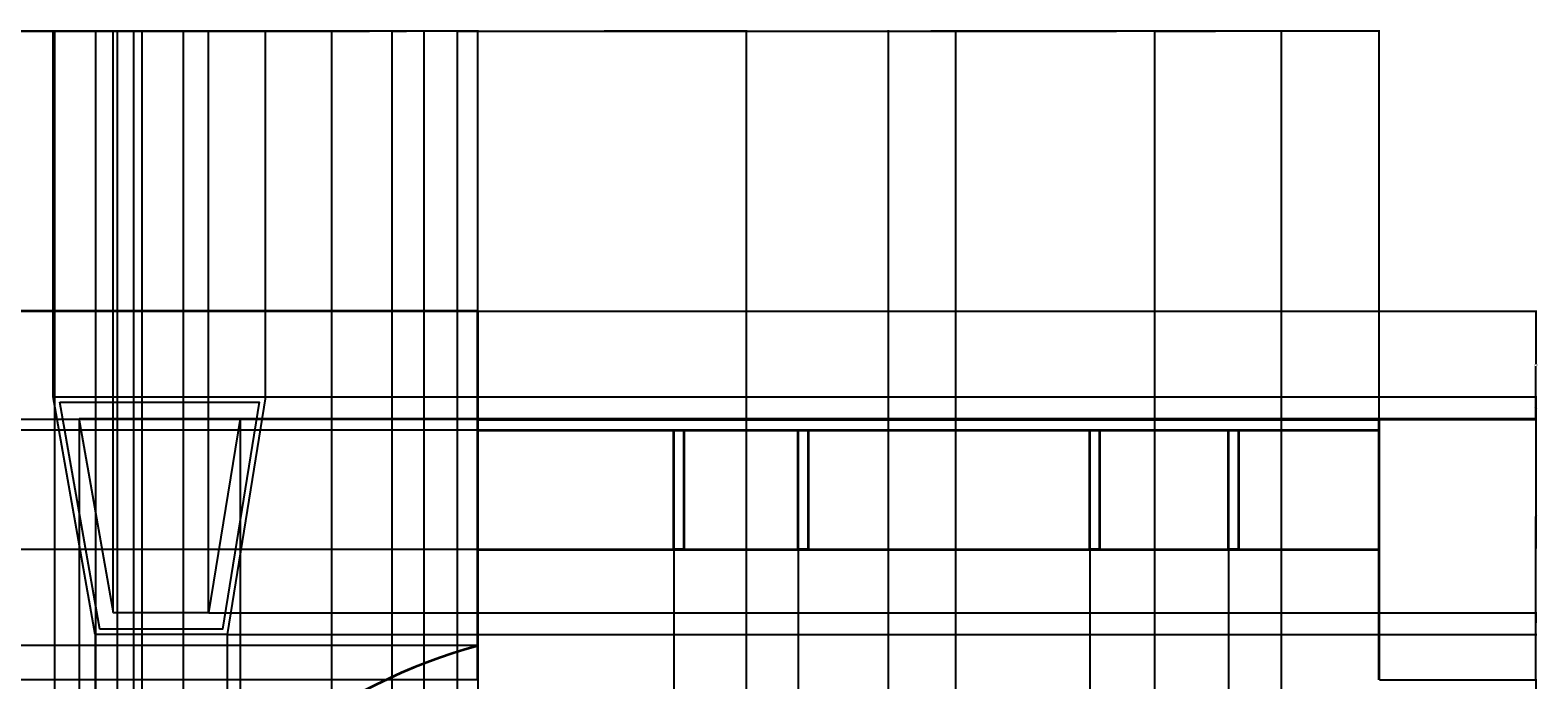
# Model space of a CAD drawing. Units: inches. Extents: x -19 to 408, y -26 to 603.
# Tile 7 of 7: x 130 to 408, y 483 to 603. Entities that reach past the tile are written whole.
import ezdxf

# ---------------------------------------------------------------- set-up
doc = ezdxf.new("R2010")
doc.units = ezdxf.units.IN
doc.header["$MEASUREMENT"] = 0
for name, color, linetype, lineweight in [('A-ANNO-DIMS', 2, 'Continuous', 18), ('A-ELEV', 7, 'Continuous', 35), ('A-GLAZ', 4, 'Continuous', 25)]:
    doc.layers.add(name, color=color, linetype=linetype, lineweight=lineweight)
doc.styles.get("Standard").update_dxf_attribs({"font": 'arial.ttf'})
doc.dimstyles.get("Standard").update_dxf_attribs({"dimtxt": 0.18, "dimasz": 0.18, "dimexe": 0.18, "dimexo": 0.0625, "dimgap": 0.09, "dimtad": 0, "dimtih": 1, "dimtoh": 1, "dimdec": 4, "dimzin": 0, "dimdsep": 46, "dimtxsty": 'Standard', "dimcen": 0.09, "dimadec": 0, "dimazin": 0, "dimtfac": 1, "dimtdec": 4, "dimtofl": 0, "dimtmove": 0, "dimatfit": 3, "dimfxl": 1, "dimtolj": 1, "dimtzin": 0, "dimarcsym": 0})

# ---------------------------------------------------------------- blocks, each defined once
blk = doc.blocks.new('RAIL-POST')
blk.add_lwpolyline([(0, 22), (1.83, 22), (1.83, 0), (0, 0)], close=True)
blk = doc.blocks.new('*D15')
at = {"layer": 'A-ANNO-DIMS', "color": 0, "lineweight": -2, "transparency": 16777216}
for p, q in [((10.2, 573.88), (10.2, 602.9)), ((10.38, 602.72), (110.85, 602.72)), ((212.25, 602.72), (111.78, 602.72)), ((212.43, 551.17), (212.43, 602.9))]:
    blk.add_line(p, q, dxfattribs=at)
at = {"layer": 'A-ANNO-DIMS', "color": 0, "transparency": 16777216}
for points in [[(10.38, 602.75), (10.38, 602.69), (10.2, 602.72)], [(212.25, 602.75), (212.25, 602.69), (212.43, 602.72)]]:
    blk.add_solid(points, dxfattribs=at)
at = {"layer": 'Defpoints', "color": 0, "transparency": 16777216}
for p in [(212.43, 602.72), (10.2, 573.82), (212.43, 551.1)]:
    blk.add_point(p, dxfattribs=at)
at = {"layer": 'A-ANNO-DIMS', "color": 0, "transparency": 16777216, "insert": (111.32, 602.72), "char_height": 0.18, "attachment_point": 5}
blk.add_mtext('\\A1;202.23', dxfattribs=at)
blk = doc.blocks.new('*D16')
at = {"layer": 'A-ANNO-DIMS', "color": 0, "lineweight": -2, "transparency": 16777216}
for p, q in [((212.43, 551.17), (212.43, 602.9)), ((212.61, 602.72), (295.05, 602.72)), ((378.39, 602.72), (295.96, 602.72)), ((378.57, 531.21), (378.57, 602.9))]:
    blk.add_line(p, q, dxfattribs=at)
at = {"layer": 'A-ANNO-DIMS', "color": 0, "transparency": 16777216}
for points in [[(212.61, 602.75), (212.61, 602.69), (212.43, 602.72)], [(378.39, 602.75), (378.39, 602.69), (378.57, 602.72)]]:
    blk.add_solid(points, dxfattribs=at)
at = {"layer": 'Defpoints', "color": 0, "transparency": 16777216}
for p in [(378.57, 602.72), (212.43, 551.1), (378.57, 531.15)]:
    blk.add_point(p, dxfattribs=at)
at = {"layer": 'A-ANNO-DIMS', "color": 0, "transparency": 16777216, "insert": (295.5, 602.72), "char_height": 0.18, "attachment_point": 5}
blk.add_mtext('\\A1;166.14', dxfattribs=at)
blk = doc.blocks.new('*D21')
at = {"layer": 'A-ANNO-DIMS', "color": 0, "lineweight": -2, "transparency": 16777216}
for p, q in [((212.37, 551.1), (-18.88, 551.1)), ((-18.7, 550.92), (-18.7, 481.31)), ((-18.7, 411.33), (-18.7, 480.94)), ((185.46, 411.15), (-18.88, 411.15))]:
    blk.add_line(p, q, dxfattribs=at)
at = {"layer": 'A-ANNO-DIMS', "color": 0, "transparency": 16777216}
for points in [[(-18.73, 550.92), (-18.67, 550.92), (-18.7, 551.1)], [(-18.73, 411.33), (-18.67, 411.33), (-18.7, 411.15)]]:
    blk.add_solid(points, dxfattribs=at)
at = {"layer": 'Defpoints', "color": 0, "transparency": 16777216}
for p in [(-18.7, 551.1), (212.43, 551.1), (185.52, 411.15)]:
    blk.add_point(p, dxfattribs=at)
at = {"layer": 'A-ANNO-DIMS', "color": 0, "transparency": 16777216, "insert": (-18.7, 481.13), "char_height": 0.18, "attachment_point": 5}
blk.add_mtext('\\A1;139.96', dxfattribs=at)
blk = doc.blocks.new('*D22')
at = {"layer": 'A-ANNO-DIMS', "color": 0, "lineweight": -2, "transparency": 16777216}
for p, q in [((10.14, 573.82), (-18.88, 573.82)), ((-18.7, 573.64), (-18.7, 562.64)), ((-18.7, 551.28), (-18.7, 562.28)), ((212.37, 551.1), (-18.88, 551.1))]:
    blk.add_line(p, q, dxfattribs=at)
at = {"layer": 'A-ANNO-DIMS', "color": 0, "transparency": 16777216}
for points in [[(-18.73, 573.64), (-18.67, 573.64), (-18.7, 573.82)], [(-18.73, 551.28), (-18.67, 551.28), (-18.7, 551.1)]]:
    blk.add_solid(points, dxfattribs=at)
at = {"layer": 'Defpoints', "color": 0, "transparency": 16777216}
for p in [(-18.7, 573.82), (10.2, 573.82), (212.43, 551.1)]:
    blk.add_point(p, dxfattribs=at)
at = {"layer": 'A-ANNO-DIMS', "color": 0, "transparency": 16777216, "insert": (-18.7, 562.46), "char_height": 0.18, "attachment_point": 5}
blk.add_mtext('\\A1;22.714', dxfattribs=at)
blk = doc.blocks.new('*D24')
at = {"layer": 'A-ANNO-DIMS', "color": 0, "lineweight": -2, "transparency": 16777216}
for p, q in [((378.63, 483.15), (407.65, 483.15)), ((407.47, 482.97), (407.47, 447.33)), ((407.47, 411.33), (407.47, 446.97)), ((360.63, 411.15), (407.65, 411.15))]:
    blk.add_line(p, q, dxfattribs=at)
at = {"layer": 'A-ANNO-DIMS', "color": 0, "transparency": 16777216}
for points in [[(407.44, 482.97), (407.5, 482.97), (407.47, 483.15)], [(407.44, 411.33), (407.5, 411.33), (407.47, 411.15)]]:
    blk.add_solid(points, dxfattribs=at)
at = {"layer": 'Defpoints', "color": 0, "transparency": 16777216}
for p in [(378.57, 483.15), (407.47, 483.15), (360.57, 411.15)]:
    blk.add_point(p, dxfattribs=at)
at = {"layer": 'A-ANNO-DIMS', "color": 0, "transparency": 16777216, "insert": (407.47, 447.15), "char_height": 0.18, "attachment_point": 5}
blk.add_mtext('\\A1;72', dxfattribs=at)
blk = doc.blocks.new('*D25')
at = {"layer": 'A-ANNO-DIMS', "color": 0, "lineweight": -2, "transparency": 16777216}
for p, q in [((378.63, 531.15), (407.65, 531.15)), ((407.47, 530.97), (407.47, 507.33)), ((407.47, 483.33), (407.47, 506.97)), ((378.63, 483.15), (407.65, 483.15))]:
    blk.add_line(p, q, dxfattribs=at)
at = {"layer": 'A-ANNO-DIMS', "color": 0, "transparency": 16777216}
for points in [[(407.44, 530.97), (407.5, 530.97), (407.47, 531.15)], [(407.44, 483.33), (407.5, 483.33), (407.47, 483.15)]]:
    blk.add_solid(points, dxfattribs=at)
at = {"layer": 'Defpoints', "color": 0, "transparency": 16777216}
for p in [(378.57, 531.15), (407.47, 531.15), (378.57, 483.15)]:
    blk.add_point(p, dxfattribs=at)
at = {"layer": 'A-ANNO-DIMS', "color": 0, "transparency": 16777216, "insert": (407.47, 507.15), "char_height": 0.18, "attachment_point": 5}
blk.add_mtext('\\A1;48', dxfattribs=at)
blk = doc.blocks.new('*D26')
at = {"layer": 'A-ANNO-DIMS', "color": 0, "lineweight": -2, "transparency": 16777216}
for p, q in [((212.49, 551.1), (407.65, 551.1)), ((407.47, 550.92), (407.47, 541.31)), ((407.47, 531.33), (407.47, 540.94)), ((378.63, 531.15), (407.65, 531.15))]:
    blk.add_line(p, q, dxfattribs=at)
at = {"layer": 'A-ANNO-DIMS', "color": 0, "transparency": 16777216}
for points in [[(407.44, 550.92), (407.5, 550.92), (407.47, 551.1)], [(407.44, 531.33), (407.5, 531.33), (407.47, 531.15)]]:
    blk.add_solid(points, dxfattribs=at)
at = {"layer": 'Defpoints', "color": 0, "transparency": 16777216}
for p in [(212.43, 551.1), (407.47, 551.1), (378.57, 531.15)]:
    blk.add_point(p, dxfattribs=at)
at = {"layer": 'A-ANNO-DIMS', "color": 0, "transparency": 16777216, "insert": (407.47, 541.13), "char_height": 0.18, "attachment_point": 5}
blk.add_mtext('\\A1;19.957', dxfattribs=at)
blk = doc.blocks.new('*D27')
at = {"layer": 'A-ANNO-DIMS', "color": 0, "lineweight": -2, "transparency": 16777216}
for p, q in [((288.17, 123.21), (288.17, 602.9)), ((288.35, 602.72), (324.05, 602.72)), ((360.39, 602.72), (324.69, 602.72)), ((360.57, 123.21), (360.57, 602.9))]:
    blk.add_line(p, q, dxfattribs=at)
at = {"layer": 'A-ANNO-DIMS', "color": 0, "transparency": 16777216}
for points in [[(288.35, 602.75), (288.35, 602.69), (288.17, 602.72)], [(360.39, 602.75), (360.39, 602.69), (360.57, 602.72)]]:
    blk.add_solid(points, dxfattribs=at)
at = {"layer": 'Defpoints', "color": 0, "transparency": 16777216}
for p in [(360.57, 602.72), (288.17, 123.15), (360.57, 123.15)]:
    blk.add_point(p, dxfattribs=at)
at = {"layer": 'A-ANNO-DIMS', "color": 0, "transparency": 16777216, "insert": (324.37, 602.72), "char_height": 0.18, "attachment_point": 5}
blk.add_mtext('\\A1;72.4', dxfattribs=at)
blk = doc.blocks.new('*D29')
at = {"layer": 'A-ANNO-DIMS', "color": 0, "lineweight": -2, "transparency": 16777216}
for p, q in [((300.56, 291.21), (300.56, 602.9)), ((300.74, 602.72), (330.19, 602.72)), ((360.39, 602.72), (330.94, 602.72)), ((360.57, 300.05), (360.57, 602.9))]:
    blk.add_line(p, q, dxfattribs=at)
at = {"layer": 'A-ANNO-DIMS', "color": 0, "transparency": 16777216}
for points in [[(300.74, 602.75), (300.74, 602.69), (300.56, 602.72)], [(360.39, 602.75), (360.39, 602.69), (360.57, 602.72)]]:
    blk.add_solid(points, dxfattribs=at)
at = {"layer": 'Defpoints', "color": 0, "transparency": 16777216}
for p in [(360.57, 602.72), (360.57, 299.99), (300.56, 291.15)]:
    blk.add_point(p, dxfattribs=at)
at = {"layer": 'A-ANNO-DIMS', "color": 0, "transparency": 16777216, "insert": (330.56, 602.72), "char_height": 0.18, "attachment_point": 5}
blk.add_mtext('\\A1;60.01', dxfattribs=at)
blk = doc.blocks.new('*D36')
at = {"layer": 'A-ANNO-DIMS', "color": 0, "lineweight": -2, "transparency": 16777216}
for p, q in [((52.15, 203.77), (52.15, 602.9)), ((52.33, 602.72), (96.69, 602.72)), ((141.84, 602.72), (97.48, 602.72)), ((142.02, 171.21), (142.02, 602.9))]:
    blk.add_line(p, q, dxfattribs=at)
at = {"layer": 'A-ANNO-DIMS', "color": 0, "transparency": 16777216}
for points in [[(52.33, 602.75), (52.33, 602.69), (52.15, 602.72)], [(141.84, 602.75), (141.84, 602.69), (142.02, 602.72)]]:
    blk.add_solid(points, dxfattribs=at)
at = {"layer": 'Defpoints', "color": 0, "transparency": 16777216}
for p in [(142.02, 602.72), (52.15, 203.7), (142.02, 171.15)]:
    blk.add_point(p, dxfattribs=at)
at = {"layer": 'A-ANNO-DIMS', "color": 0, "transparency": 16777216, "insert": (97.09, 602.72), "char_height": 0.18, "attachment_point": 5}
blk.add_mtext('\\A1;89.87', dxfattribs=at)
blk = doc.blocks.new('*D37')
at = {"layer": 'A-ANNO-DIMS', "color": 0, "lineweight": -2, "transparency": 16777216}
for p, q in [((142.02, 171.21), (142.02, 602.9)), ((142.2, 602.72), (174.97, 602.72)), ((208.53, 602.72), (175.76, 602.72)), ((208.71, 171.21), (208.71, 602.9))]:
    blk.add_line(p, q, dxfattribs=at)
at = {"layer": 'A-ANNO-DIMS', "color": 0, "transparency": 16777216}
for points in [[(142.2, 602.75), (142.2, 602.69), (142.02, 602.72)], [(208.53, 602.75), (208.53, 602.69), (208.71, 602.72)]]:
    blk.add_solid(points, dxfattribs=at)
at = {"layer": 'Defpoints', "color": 0, "transparency": 16777216}
for p in [(208.71, 602.72), (142.02, 171.15), (208.71, 171.15)]:
    blk.add_point(p, dxfattribs=at)
at = {"layer": 'A-ANNO-DIMS', "color": 0, "transparency": 16777216, "insert": (175.37, 602.72), "char_height": 0.18, "attachment_point": 5}
blk.add_mtext('\\A1;66.69', dxfattribs=at)
blk = doc.blocks.new('*D38')
at = {"layer": 'A-ANNO-DIMS', "color": 0, "lineweight": -2, "transparency": 16777216}
for p, q in [((208.71, 171.21), (208.71, 602.9)), ((208.89, 602.72), (234.95, 602.72)), ((261.81, 602.72), (235.74, 602.72)), ((261.99, 203.77), (261.99, 602.9))]:
    blk.add_line(p, q, dxfattribs=at)
at = {"layer": 'A-ANNO-DIMS', "color": 0, "transparency": 16777216}
for points in [[(208.89, 602.75), (208.89, 602.69), (208.71, 602.72)], [(261.81, 602.75), (261.81, 602.69), (261.99, 602.72)]]:
    blk.add_solid(points, dxfattribs=at)
at = {"layer": 'Defpoints', "color": 0, "transparency": 16777216}
for p in [(261.99, 602.72), (261.99, 203.7), (208.71, 171.15)]:
    blk.add_point(p, dxfattribs=at)
at = {"layer": 'A-ANNO-DIMS', "color": 0, "transparency": 16777216, "insert": (235.35, 602.72), "char_height": 0.18, "attachment_point": 5}
blk.add_mtext('\\A1;53.28', dxfattribs=at)
blk = doc.blocks.new('*D45')
at = {"layer": 'A-ANNO-DIMS', "color": 0, "lineweight": -2, "transparency": 16777216}
for p, q in [((36.57, 219.21), (36.57, 602.9)), ((36.75, 602.72), (85.2, 602.72)), ((134.3, 602.72), (85.85, 602.72)), ((134.48, 220.21), (134.48, 602.9))]:
    blk.add_line(p, q, dxfattribs=at)
at = {"layer": 'A-ANNO-DIMS', "color": 0, "transparency": 16777216}
for points in [[(36.75, 602.75), (36.75, 602.69), (36.57, 602.72)], [(134.3, 602.75), (134.3, 602.69), (134.48, 602.72)]]:
    blk.add_solid(points, dxfattribs=at)
at = {"layer": 'Defpoints', "color": 0, "transparency": 16777216}
for p in [(134.48, 602.72), (134.48, 220.15), (36.57, 219.15)]:
    blk.add_point(p, dxfattribs=at)
at = {"layer": 'A-ANNO-DIMS', "color": 0, "transparency": 16777216, "insert": (85.52, 602.72), "char_height": 0.18, "attachment_point": 5}
blk.add_mtext('\\A1;97.9', dxfattribs=at)
blk = doc.blocks.new('*D46')
at = {"layer": 'A-ANNO-DIMS', "color": 0, "lineweight": -2, "transparency": 16777216}
for p, q in [((337.23, 171.21), (337.23, 602.9)), ((337.41, 602.72), (348.43, 602.72)), ((360.39, 602.72), (349.36, 602.72)), ((360.57, 173.74), (360.57, 602.9))]:
    blk.add_line(p, q, dxfattribs=at)
at = {"layer": 'A-ANNO-DIMS', "color": 0, "transparency": 16777216}
for points in [[(337.41, 602.75), (337.41, 602.69), (337.23, 602.72)], [(360.39, 602.75), (360.39, 602.69), (360.57, 602.72)]]:
    blk.add_solid(points, dxfattribs=at)
at = {"layer": 'Defpoints', "color": 0, "transparency": 16777216}
for p in [(360.57, 602.72), (360.57, 173.67), (337.23, 171.15)]:
    blk.add_point(p, dxfattribs=at)
at = {"layer": 'A-ANNO-DIMS', "color": 0, "transparency": 16777216, "insert": (348.9, 602.72), "char_height": 0.18, "attachment_point": 5}
blk.add_mtext('\\A1;23.345', dxfattribs=at)
blk = doc.blocks.new('*D55')
at = {"layer": 'A-ANNO-DIMS', "color": 0, "lineweight": -2, "transparency": 16777216}
for p, q in [((146.02, 199.77), (146.02, 602.9)), ((146.2, 602.72), (147.14, 602.72)), ((148.87, 602.72), (147.93, 602.72)), ((149.05, 196.37), (149.05, 602.9))]:
    blk.add_line(p, q, dxfattribs=at)
at = {"layer": 'A-ANNO-DIMS', "color": 0, "transparency": 16777216}
for points in [[(146.2, 602.75), (146.2, 602.69), (146.02, 602.72)], [(148.87, 602.75), (148.87, 602.69), (149.05, 602.72)]]:
    blk.add_solid(points, dxfattribs=at)
at = {"layer": 'Defpoints', "color": 0, "transparency": 16777216}
for p in [(149.05, 602.72), (146.02, 199.7), (149.05, 196.31)]:
    blk.add_point(p, dxfattribs=at)
at = {"layer": 'A-ANNO-DIMS', "color": 0, "transparency": 16777216, "insert": (147.54, 602.72), "char_height": 0.18, "attachment_point": 5}
blk.add_mtext('\\A1;3.029', dxfattribs=at)
blk = doc.blocks.new('*D56')
at = {"layer": 'A-ANNO-DIMS', "color": 0, "lineweight": -2, "transparency": 16777216}
for p, q in [((149.05, 196.37), (149.05, 602.9)), ((149.23, 602.72), (153.3, 602.72)), ((158.02, 602.72), (153.95, 602.72)), ((158.2, 196.37), (158.2, 602.9))]:
    blk.add_line(p, q, dxfattribs=at)
at = {"layer": 'A-ANNO-DIMS', "color": 0, "transparency": 16777216}
for points in [[(149.23, 602.75), (149.23, 602.69), (149.05, 602.72)], [(158.02, 602.75), (158.02, 602.69), (158.2, 602.72)]]:
    blk.add_solid(points, dxfattribs=at)
at = {"layer": 'Defpoints', "color": 0, "transparency": 16777216}
for p in [(158.2, 602.72), (149.05, 196.31), (158.2, 196.31)]:
    blk.add_point(p, dxfattribs=at)
at = {"layer": 'A-ANNO-DIMS', "color": 0, "transparency": 16777216, "insert": (153.63, 602.72), "char_height": 0.18, "attachment_point": 5}
blk.add_mtext('\\A1;9.15', dxfattribs=at)
blk = doc.blocks.new('*D74')
at = {"layer": 'A-ANNO-DIMS', "color": 0, "lineweight": -2, "transparency": 16777216}
for p, q in [((208.71, 411.21), (208.71, 602.9)), ((208.89, 602.72), (234.95, 602.72)), ((261.81, 602.72), (235.74, 602.72)), ((261.99, 443.77), (261.99, 602.9))]:
    blk.add_line(p, q, dxfattribs=at)
at = {"layer": 'A-ANNO-DIMS', "color": 0, "transparency": 16777216}
for points in [[(208.89, 602.75), (208.89, 602.69), (208.71, 602.72)], [(261.81, 602.75), (261.81, 602.69), (261.99, 602.72)]]:
    blk.add_solid(points, dxfattribs=at)
at = {"layer": 'Defpoints', "color": 0, "transparency": 16777216}
for p in [(261.99, 602.72), (261.99, 443.7), (208.71, 411.15)]:
    blk.add_point(p, dxfattribs=at)
at = {"layer": 'A-ANNO-DIMS', "color": 0, "transparency": 16777216, "insert": (235.35, 602.72), "char_height": 0.18, "attachment_point": 5}
blk.add_mtext('\\A1;53.28', dxfattribs=at)
blk = doc.blocks.new('*D75')
at = {"layer": 'A-ANNO-DIMS', "color": 0, "lineweight": -2, "transparency": 16777216}
for p, q in [((212.43, 507.08), (212.43, -25.93)), ((248.57, 507.08), (248.57, -25.93)), ((212.61, -25.75), (230.11, -25.75)), ((248.39, -25.75), (230.89, -25.75))]:
    blk.add_line(p, q, dxfattribs=at)
at = {"layer": 'A-ANNO-DIMS', "color": 0, "transparency": 16777216}
for points in [[(212.61, -25.72), (212.61, -25.78), (212.43, -25.75)], [(248.39, -25.72), (248.39, -25.78), (248.57, -25.75)]]:
    blk.add_solid(points, dxfattribs=at)
at = {"layer": 'Defpoints', "color": 0, "transparency": 16777216}
for p in [(212.43, 507.15), (248.57, 507.15), (248.57, -25.75)]:
    blk.add_point(p, dxfattribs=at)
at = {"layer": 'A-ANNO-DIMS', "color": 0, "transparency": 16777216, "insert": (230.5, -25.75), "char_height": 0.18, "attachment_point": 5}
blk.add_mtext('\\A1;36.14', dxfattribs=at)
blk = doc.blocks.new('*D76')
at = {"layer": 'A-ANNO-DIMS', "color": 0, "lineweight": -2, "transparency": 16777216}
for p, q in [((248.57, 507.08), (248.57, -25.93)), ((271.51, 507.08), (271.51, -25.93)), ((248.75, -25.75), (259.58, -25.75)), ((271.33, -25.75), (260.51, -25.75))]:
    blk.add_line(p, q, dxfattribs=at)
at = {"layer": 'A-ANNO-DIMS', "color": 0, "transparency": 16777216}
for points in [[(248.75, -25.72), (248.75, -25.78), (248.57, -25.75)], [(271.33, -25.72), (271.33, -25.78), (271.51, -25.75)]]:
    blk.add_solid(points, dxfattribs=at)
at = {"layer": 'Defpoints', "color": 0, "transparency": 16777216}
for p in [(248.57, 507.15), (271.51, 507.15), (271.51, -25.75)]:
    blk.add_point(p, dxfattribs=at)
at = {"layer": 'A-ANNO-DIMS', "color": 0, "transparency": 16777216, "insert": (260.04, -25.75), "char_height": 0.18, "attachment_point": 5}
blk.add_mtext('\\A1;22.944', dxfattribs=at)
blk = doc.blocks.new('*D77')
at = {"layer": 'A-ANNO-DIMS', "color": 0, "lineweight": -2, "transparency": 16777216}
for p, q in [((271.51, 507.08), (271.51, -25.93)), ((325.24, 507.08), (325.24, -25.93)), ((271.69, -25.75), (297.98, -25.75)), ((325.06, -25.75), (298.77, -25.75))]:
    blk.add_line(p, q, dxfattribs=at)
at = {"layer": 'A-ANNO-DIMS', "color": 0, "transparency": 16777216}
for points in [[(271.69, -25.72), (271.69, -25.78), (271.51, -25.75)], [(325.06, -25.72), (325.06, -25.78), (325.24, -25.75)]]:
    blk.add_solid(points, dxfattribs=at)
at = {"layer": 'Defpoints', "color": 0, "transparency": 16777216}
for p in [(271.51, 507.15), (325.24, 507.15), (325.24, -25.75)]:
    blk.add_point(p, dxfattribs=at)
at = {"layer": 'A-ANNO-DIMS', "color": 0, "transparency": 16777216, "insert": (298.38, -25.75), "char_height": 0.18, "attachment_point": 5}
blk.add_mtext('\\A1;53.72', dxfattribs=at)
blk = doc.blocks.new('*D78')
at = {"layer": 'A-ANNO-DIMS', "color": 0, "lineweight": -2, "transparency": 16777216}
for p, q in [((325.24, 507.08), (325.24, -25.93)), ((350.82, 507.08), (350.82, -25.93)), ((325.42, -25.75), (337.56, -25.75)), ((350.64, -25.75), (338.49, -25.75))]:
    blk.add_line(p, q, dxfattribs=at)
at = {"layer": 'A-ANNO-DIMS', "color": 0, "transparency": 16777216}
for points in [[(325.42, -25.72), (325.42, -25.78), (325.24, -25.75)], [(350.64, -25.72), (350.64, -25.78), (350.82, -25.75)]]:
    blk.add_solid(points, dxfattribs=at)
at = {"layer": 'Defpoints', "color": 0, "transparency": 16777216}
for p in [(325.24, 507.15), (350.82, 507.15), (350.82, -25.75)]:
    blk.add_point(p, dxfattribs=at)
at = {"layer": 'A-ANNO-DIMS', "color": 0, "transparency": 16777216, "insert": (338.03, -25.75), "char_height": 0.18, "attachment_point": 5}
blk.add_mtext('\\A1;25.584', dxfattribs=at)
blk = doc.blocks.new('*D79')
at = {"layer": 'A-ANNO-DIMS', "color": 0, "lineweight": -2, "transparency": 16777216}
for p, q in [((212.37, 489.45), (-18.88, 489.45)), ((-18.7, 489.27), (-18.7, 486.48)), ((-18.7, 483.33), (-18.7, 486.12)), ((212.37, 483.15), (-18.88, 483.15))]:
    blk.add_line(p, q, dxfattribs=at)
at = {"layer": 'A-ANNO-DIMS', "color": 0, "transparency": 16777216}
for points in [[(-18.73, 489.27), (-18.67, 489.27), (-18.7, 489.45)], [(-18.73, 483.33), (-18.67, 483.33), (-18.7, 483.15)]]:
    blk.add_solid(points, dxfattribs=at)
at = {"layer": 'Defpoints', "color": 0, "transparency": 16777216}
for p in [(-18.7, 489.45), (212.43, 489.45), (212.43, 483.15)]:
    blk.add_point(p, dxfattribs=at)
at = {"layer": 'A-ANNO-DIMS', "color": 0, "transparency": 16777216, "insert": (-18.7, 486.3), "char_height": 0.18, "attachment_point": 5}
blk.add_mtext('\\A1;6.3', dxfattribs=at)
blk = doc.blocks.new('*D80')
at = {"layer": 'A-ANNO-DIMS', "color": 0, "lineweight": -2, "transparency": 16777216}
for p, q in [((212.37, 507.15), (-18.88, 507.15)), ((-18.7, 506.97), (-18.7, 495.33)), ((-18.7, 483.33), (-18.7, 494.97)), ((212.37, 483.15), (-18.88, 483.15))]:
    blk.add_line(p, q, dxfattribs=at)
at = {"layer": 'A-ANNO-DIMS', "color": 0, "transparency": 16777216}
for points in [[(-18.73, 506.97), (-18.67, 506.97), (-18.7, 507.15)], [(-18.73, 483.33), (-18.67, 483.33), (-18.7, 483.15)]]:
    blk.add_solid(points, dxfattribs=at)
at = {"layer": 'Defpoints', "color": 0, "transparency": 16777216}
for p in [(-18.7, 507.15), (212.43, 507.15), (212.43, 483.15)]:
    blk.add_point(p, dxfattribs=at)
at = {"layer": 'A-ANNO-DIMS', "color": 0, "transparency": 16777216, "insert": (-18.7, 495.15), "char_height": 0.18, "attachment_point": 5}
blk.add_mtext('\\A1;24', dxfattribs=at)
blk = doc.blocks.new('*D81')
at = {"layer": 'A-ANNO-DIMS', "color": 0, "lineweight": -2, "transparency": 16777216}
for p, q in [((212.37, 531.15), (-18.88, 531.15)), ((-18.7, 530.97), (-18.7, 530.33)), ((212.37, 529.15), (-18.88, 529.15)), ((-18.7, 529.33), (-18.7, 529.97))]:
    blk.add_line(p, q, dxfattribs=at)
at = {"layer": 'A-ANNO-DIMS', "color": 0, "transparency": 16777216}
for points in [[(-18.73, 530.97), (-18.67, 530.97), (-18.7, 531.15)], [(-18.73, 529.33), (-18.67, 529.33), (-18.7, 529.15)]]:
    blk.add_solid(points, dxfattribs=at)
at = {"layer": 'Defpoints', "color": 0, "transparency": 16777216}
for p in [(-18.7, 531.15), (212.43, 531.15), (212.43, 529.15)]:
    blk.add_point(p, dxfattribs=at)
at = {"layer": 'A-ANNO-DIMS', "color": 0, "transparency": 16777216, "insert": (-18.7, 530.15), "char_height": 0.18, "attachment_point": 5}
blk.add_mtext('\\A1;2', dxfattribs=at)
blk = doc.blocks.new('*D82')
at = {"layer": 'A-ANNO-DIMS', "color": 0, "lineweight": -2, "transparency": 16777216}
for p, q in [((134.21, 535.4), (134.21, 602.9)), ((134.39, 602.72), (153.31, 602.72)), ((173.16, 602.72), (154.24, 602.72)), ((173.34, 535.4), (173.34, 602.9))]:
    blk.add_line(p, q, dxfattribs=at)
at = {"layer": 'A-ANNO-DIMS', "color": 0, "transparency": 16777216}
for points in [[(134.39, 602.75), (134.39, 602.69), (134.21, 602.72)], [(173.16, 602.75), (173.16, 602.69), (173.34, 602.72)]]:
    blk.add_solid(points, dxfattribs=at)
at = {"layer": 'Defpoints', "color": 0, "transparency": 16777216}
for p in [(173.34, 602.72), (134.21, 535.34), (173.34, 535.34)]:
    blk.add_point(p, dxfattribs=at)
at = {"layer": 'A-ANNO-DIMS', "color": 0, "transparency": 16777216, "insert": (153.78, 602.72), "char_height": 0.18, "attachment_point": 5}
blk.add_mtext('\\A1;39.136', dxfattribs=at)
blk = doc.blocks.new('*D83')
at = {"layer": 'A-ANNO-DIMS', "color": 0, "lineweight": -2, "transparency": 16777216}
for p, q in [((141.92, 491.44), (141.92, -25.93)), ((166.23, 491.44), (166.23, -25.93)), ((142.1, -25.75), (153.69, -25.75)), ((166.05, -25.75), (154.45, -25.75))]:
    blk.add_line(p, q, dxfattribs=at)
at = {"layer": 'A-ANNO-DIMS', "color": 0, "transparency": 16777216}
for points in [[(142.1, -25.72), (142.1, -25.78), (141.92, -25.75)], [(166.05, -25.72), (166.05, -25.78), (166.23, -25.75)]]:
    blk.add_solid(points, dxfattribs=at)
at = {"layer": 'Defpoints', "color": 0, "transparency": 16777216}
for p in [(141.92, 491.5), (166.23, 491.5), (166.23, -25.75)]:
    blk.add_point(p, dxfattribs=at)
at = {"layer": 'A-ANNO-DIMS', "color": 0, "transparency": 16777216, "insert": (154.07, -25.75), "char_height": 0.18, "attachment_point": 5}
blk.add_mtext('\\A1;24.31', dxfattribs=at)
blk = doc.blocks.new('*D84')
at = {"layer": 'A-ANNO-DIMS', "color": 0, "lineweight": -2, "transparency": 16777216}
for p, q in [((138.97, 531.28), (138.97, -25.93)), ((168.64, 531.28), (168.64, -25.93)), ((139.15, -25.75), (153.41, -25.75)), ((168.46, -25.75), (154.2, -25.75))]:
    blk.add_line(p, q, dxfattribs=at)
at = {"layer": 'A-ANNO-DIMS', "color": 0, "transparency": 16777216}
for points in [[(139.15, -25.72), (139.15, -25.78), (138.97, -25.75)], [(168.46, -25.72), (168.46, -25.78), (168.64, -25.75)]]:
    blk.add_solid(points, dxfattribs=at)
at = {"layer": 'Defpoints', "color": 0, "transparency": 16777216}
for p in [(138.97, 531.34), (168.64, 531.34), (168.64, -25.75)]:
    blk.add_point(p, dxfattribs=at)
at = {"layer": 'A-ANNO-DIMS', "color": 0, "transparency": 16777216, "insert": (153.81, -25.75), "char_height": 0.18, "attachment_point": 5}
blk.add_mtext('\\A1;29.67', dxfattribs=at)
blk = doc.blocks.new('*D85')
at = {"layer": 'A-ANNO-DIMS', "color": 0, "lineweight": -2, "transparency": 16777216}
for p, q in [((145.27, 495.57), (145.27, 602.9)), ((145.45, 602.72), (153.66, 602.72)), ((162.64, 602.72), (154.44, 602.72)), ((162.82, 495.57), (162.82, 602.9))]:
    blk.add_line(p, q, dxfattribs=at)
at = {"layer": 'A-ANNO-DIMS', "color": 0, "transparency": 16777216}
for points in [[(145.45, 602.75), (145.45, 602.69), (145.27, 602.72)], [(162.64, 602.75), (162.64, 602.69), (162.82, 602.72)]]:
    blk.add_solid(points, dxfattribs=at)
at = {"layer": 'Defpoints', "color": 0, "transparency": 16777216}
for p in [(162.82, 602.72), (145.27, 495.5), (162.82, 495.5)]:
    blk.add_point(p, dxfattribs=at)
at = {"layer": 'A-ANNO-DIMS', "color": 0, "transparency": 16777216, "insert": (154.05, 602.72), "char_height": 0.18, "attachment_point": 5}
blk.add_mtext('\\A1;17.55', dxfattribs=at)
blk = doc.blocks.new('*D86')
at = {"layer": 'A-ANNO-DIMS', "color": 0, "lineweight": -2, "transparency": 16777216}
for p, q in [((173.41, 535.34), (407.65, 535.34)), ((407.47, 535.16), (407.47, 513.6)), ((407.47, 491.68), (407.47, 513.24)), ((166.29, 491.5), (407.65, 491.5))]:
    blk.add_line(p, q, dxfattribs=at)
at = {"layer": 'A-ANNO-DIMS', "color": 0, "transparency": 16777216}
for points in [[(407.44, 535.16), (407.5, 535.16), (407.47, 535.34)], [(407.44, 491.68), (407.5, 491.68), (407.47, 491.5)]]:
    blk.add_solid(points, dxfattribs=at)
at = {"layer": 'Defpoints', "color": 0, "transparency": 16777216}
for p in [(173.34, 535.34), (166.23, 491.5), (407.47, 491.5)]:
    blk.add_point(p, dxfattribs=at)
at = {"layer": 'A-ANNO-DIMS', "color": 0, "transparency": 16777216, "insert": (407.47, 513.42), "char_height": 0.18, "attachment_point": 5}
blk.add_mtext('\\A1;43.84', dxfattribs=at)
blk = doc.blocks.new('*D87')
at = {"layer": 'A-ANNO-DIMS', "color": 0, "lineweight": -2, "transparency": 16777216}
for p, q in [((173.406187, 535.342106), (407.651202, 535.342106)), ((407.471202, 535.162106), (407.471202, 533.522106)), ((168.704577, 531.342106), (407.651202, 531.342106)), ((407.471202, 531.522106), (407.471202, 533.162106))]:
    blk.add_line(p, q, dxfattribs=at)
at = {"layer": 'A-ANNO-DIMS', "color": 0, "transparency": 16777216}
for points in [[(407.441202, 535.162106), (407.501202, 535.162106), (407.471202, 535.342106)], [(407.441202, 531.522106), (407.501202, 531.522106), (407.471202, 531.342106)]]:
    blk.add_solid(points, dxfattribs=at)
at = {"layer": 'Defpoints', "color": 0, "transparency": 16777216}
for p in [(173.343687, 535.342106), (407.471202, 535.342106), (168.642077, 531.342106)]:
    blk.add_point(p, dxfattribs=at)
at = {"layer": 'A-ANNO-DIMS', "color": 0, "transparency": 16777216, "insert": (407.471202, 533.342106), "char_height": 0.18, "attachment_point": 5}
blk.add_mtext('\\A1;4', dxfattribs=at)
blk = doc.blocks.new('*D88')
at = {"layer": 'A-ANNO-DIMS', "color": 0, "lineweight": -2, "transparency": 16777216}
for p, q in [((162.887457, 495.503657), (407.651202, 495.503657)), ((407.471202, 495.323657), (407.471202, 493.683657)), ((407.471202, 491.683657), (407.471202, 493.323657)), ((166.290547, 491.503657), (407.651202, 491.503657))]:
    blk.add_line(p, q, dxfattribs=at)
at = {"layer": 'A-ANNO-DIMS', "color": 0, "transparency": 16777216}
for points in [[(407.441202, 495.323657), (407.501202, 495.323657), (407.471202, 495.503657)], [(407.441202, 491.683657), (407.501202, 491.683657), (407.471202, 491.503657)]]:
    blk.add_solid(points, dxfattribs=at)
at = {"layer": 'Defpoints', "color": 0, "transparency": 16777216}
for p in [(162.824957, 495.503657), (166.228047, 491.503657), (407.471202, 491.503657)]:
    blk.add_point(p, dxfattribs=at)
at = {"layer": 'A-ANNO-DIMS', "color": 0, "transparency": 16777216, "insert": (407.471202, 493.503657), "char_height": 0.18, "attachment_point": 5}
blk.add_mtext('\\A1;4', dxfattribs=at)
blk = doc.blocks.new('*D89')
at = {"layer": 'A-ANNO-DIMS', "color": 0, "lineweight": -2, "transparency": 16777216}
for p, q in [((173.34, 535.4), (173.34, 602.9)), ((173.52, 602.72), (192.49, 602.72)), ((212.25, 602.72), (193.28, 602.72)), ((212.43, 531.21), (212.43, 602.9))]:
    blk.add_line(p, q, dxfattribs=at)
at = {"layer": 'A-ANNO-DIMS', "color": 0, "transparency": 16777216}
for points in [[(173.52, 602.75), (173.52, 602.69), (173.34, 602.72)], [(212.25, 602.75), (212.25, 602.69), (212.43, 602.72)]]:
    blk.add_solid(points, dxfattribs=at)
at = {"layer": 'Defpoints', "color": 0, "transparency": 16777216}
for p in [(212.43, 602.72), (173.34, 535.34), (212.43, 531.15)]:
    blk.add_point(p, dxfattribs=at)
at = {"layer": 'A-ANNO-DIMS', "color": 0, "transparency": 16777216, "insert": (192.89, 602.72), "char_height": 0.18, "attachment_point": 5}
blk.add_mtext('\\A1;39.09', dxfattribs=at)
blk = doc.blocks.new('*D90')
at = {"layer": 'A-ANNO-DIMS', "color": 0, "lineweight": -2, "transparency": 16777216}
for p, q in [((173.41, 535.34), (407.65, 535.34)), ((407.47, 535.16), (407.47, 533.43)), ((212.49, 531.15), (407.65, 531.15)), ((407.47, 531.33), (407.47, 533.06))]:
    blk.add_line(p, q, dxfattribs=at)
at = {"layer": 'A-ANNO-DIMS', "color": 0, "transparency": 16777216}
for points in [[(407.44, 535.16), (407.5, 535.16), (407.47, 535.34)], [(407.44, 531.33), (407.5, 531.33), (407.47, 531.15)]]:
    blk.add_solid(points, dxfattribs=at)
at = {"layer": 'Defpoints', "color": 0, "transparency": 16777216}
for p in [(173.34, 535.34), (212.43, 531.15), (407.47, 531.15)]:
    blk.add_point(p, dxfattribs=at)
at = {"layer": 'A-ANNO-DIMS', "color": 0, "transparency": 16777216, "insert": (407.47, 533.24), "char_height": 0.18, "attachment_point": 5}
blk.add_mtext('\\A1;4.195', dxfattribs=at)
blk = doc.blocks.new('*D95')
at = {"layer": 'A-ANNO-DIMS', "color": 0, "lineweight": -2, "transparency": 16777216}
for p, q in [((150.57, 85.97), (150.57, 602.9)), ((150.75, 602.72), (173.31, 602.72)), ((196.49, 602.72), (173.93, 602.72)), ((196.67, 85.97), (196.67, 602.9))]:
    blk.add_line(p, q, dxfattribs=at)
at = {"layer": 'A-ANNO-DIMS', "color": 0, "transparency": 16777216}
for points in [[(150.75, 602.75), (150.75, 602.69), (150.57, 602.72)], [(196.49, 602.75), (196.49, 602.69), (196.67, 602.72)]]:
    blk.add_solid(points, dxfattribs=at)
at = {"layer": 'Defpoints', "color": 0, "transparency": 16777216}
for p in [(196.67, 602.72), (150.57, 85.9), (196.67, 85.9)]:
    blk.add_point(p, dxfattribs=at)
at = {"layer": 'A-ANNO-DIMS', "color": 0, "transparency": 16777216, "insert": (173.62, 602.72), "char_height": 0.18, "attachment_point": 5}
blk.add_mtext('\\A1;46.1', dxfattribs=at)
blk = doc.blocks.new('*D96')
at = {"layer": 'A-ANNO-DIMS', "color": 0, "lineweight": -2, "transparency": 16777216}
for p, q in [((196.67, 85.97), (196.67, 602.9)), ((196.85, 602.72), (199.31, 602.72)), ((202.41, 602.72), (199.96, 602.72)), ((202.59, 85.97), (202.59, 602.9))]:
    blk.add_line(p, q, dxfattribs=at)
at = {"layer": 'A-ANNO-DIMS', "color": 0, "transparency": 16777216}
for points in [[(196.85, 602.75), (196.85, 602.69), (196.67, 602.72)], [(202.41, 602.75), (202.41, 602.69), (202.59, 602.72)]]:
    blk.add_solid(points, dxfattribs=at)
at = {"layer": 'Defpoints', "color": 0, "transparency": 16777216}
for p in [(202.59, 602.72), (196.67, 85.9), (202.59, 85.9)]:
    blk.add_point(p, dxfattribs=at)
at = {"layer": 'A-ANNO-DIMS', "color": 0, "transparency": 16777216, "insert": (199.63, 602.72), "char_height": 0.18, "attachment_point": 5}
blk.add_mtext('\\A1;5.92', dxfattribs=at)
blk = doc.blocks.new('*D105')
at = {"layer": 'A-ANNO-DIMS', "color": 0, "lineweight": -2, "transparency": 16777216}
for p, q in [((120.05, 411.21), (120.05, 602.9)), ((120.23, 602.72), (152.39, 602.72)), ((185.34, 602.72), (153.18, 602.72)), ((185.52, 411.21), (185.52, 602.9))]:
    blk.add_line(p, q, dxfattribs=at)
at = {"layer": 'A-ANNO-DIMS', "color": 0, "transparency": 16777216}
for points in [[(120.23, 602.75), (120.23, 602.69), (120.05, 602.72)], [(185.34, 602.75), (185.34, 602.69), (185.52, 602.72)]]:
    blk.add_solid(points, dxfattribs=at)
at = {"layer": 'Defpoints', "color": 0, "transparency": 16777216}
for p in [(120.05, 602.72), (120.05, 411.15), (185.52, 411.15)]:
    blk.add_point(p, dxfattribs=at)
at = {"layer": 'A-ANNO-DIMS', "color": 0, "transparency": 16777216, "insert": (152.79, 602.72), "char_height": 0.18, "attachment_point": 5}
blk.add_mtext('\\A1;65.47', dxfattribs=at)

msp = doc.modelspace()

# ---------------------------------------------------------------- linework, layer by layer
at = {"layer": 'A-ELEV'}
for p, q in [((212.4303, 551.1043), (41.4148, 551.1043)), ((212.4303, 483.1472), (212.4303, 551.1043)), ((212.4303, 531.1472), (378.5712, 531.1472)), ((378.5712, 483.1472), (378.5712, 531.1472)), ((212.4303, 529.1472), (378.5712, 529.1472)), ((212.4303, 507.1472), (378.5712, 507.1472))]:
    msp.add_line(p, q, dxfattribs=at)
msp.add_ellipse((188.4962, 355.8525), major_axis=(71.2607, 129.8447), ratio=0.58959924, start_param=6.80188927, end_param=9.63162337, dxfattribs=at)
at = {"layer": 'A-GLAZ'}
for points in [[(134.2076, 535.3421), (173.3437, 535.3421), (166.228, 491.5037), (141.9163, 491.5037)], [(135.3988, 534.3421), (172.1683, 534.3421), (165.3773, 492.5037), (142.7558, 492.5037)], [(138.9724, 531.3421), (168.6421, 531.3421), (162.825, 495.5037), (145.2743, 495.5037)]]:
    msp.add_lwpolyline(points, close=True, dxfattribs=at)

# ---------------------------------------------------------------- block references
at = {"layer": 'A-ELEV'}
for p in [(248.5701, 507.147), (271.5138, 507.147), (325.2364, 507.147), (350.8207, 507.147)]:
    msp.add_blockref('RAIL-POST', p, dxfattribs=at)

# ---------------------------------------------------------------- dimensions: what is measured, and where the dimension line sits
at = {"layer": 'A-ANNO-DIMS'}
for base, p1, p2, override, picture, middle in [((212.4303, 602.7184), (10.202, 573.8184), (212.4303, 551.1043), {"dimdec": 2, "dimlfac": 1, "dimrnd": 0, "dimzin": 0, "dimdsep": 46, "dimlunit": 2}, '*D15', (111.3162, 602.7184)), ((134.4772, 602.7184), (36.5712, 219.1472), (134.4772, 220.1467), {"dimdec": 1, "dimlfac": 1, "dimrnd": 0, "dimzin": 0, "dimdsep": 46, "dimlunit": 2}, '*D45', (85.5242, 602.7184)), ((142.0243, 602.7184), (52.1528, 203.704), (142.0243, 171.1472), {"dimdec": 2, "dimlfac": 1, "dimrnd": 0, "dimzin": 0, "dimdsep": 46, "dimlunit": 2}, '*D36', (97.0885, 602.7184)), ((120.0489, 602.7184), (185.5212, 411.1472), (120.0489, 411.1472), {"dimdec": 2, "dimlfac": 1, "dimrnd": 0, "dimzin": 0, "dimdsep": 46, "dimlunit": 2}, '*D105', (152.7851, 602.7184)), ((173.3437, 602.7184), (134.2076, 535.3421), (173.3437, 535.3421), {"dimdec": 3, "dimlfac": 1, "dimrnd": 0, "dimzin": 0, "dimdsep": 46, "dimlunit": 2}, '*D82', (153.7757, 602.7184)), ((208.70929, 602.71845), (142.02426, 171.14723), (208.70929, 171.14723), {"dimdec": 2, "dimlfac": 1, "dimrnd": 0, "dimzin": 0, "dimdsep": 46, "dimlunit": 2}, '*D37', (175.36677, 602.71845)), ((162.825, 602.7184), (145.2743, 495.5037), (162.825, 495.5037), {"dimdec": 2, "dimlfac": 1, "dimrnd": 0, "dimzin": 0, "dimdsep": 46, "dimlunit": 2}, '*D85', (154.0496, 602.7184)), ((149.0532, 602.7184), (146.0243, 199.704), (149.0532, 196.3059), {"dimdec": 3, "dimlfac": 1, "dimrnd": 0, "dimzin": 0, "dimdsep": 46, "dimlunit": 2}, '*D55', (147.5387, 602.7184)), ((158.2025, 602.7184), (149.0532, 196.3059), (158.2025, 196.3059), {"dimdec": 2, "dimlfac": 1, "dimrnd": 0, "dimzin": 0, "dimdsep": 46, "dimlunit": 2}, '*D56', (153.6278, 602.7184)), ((196.6731, 602.7184), (150.5712, 85.9033), (196.6731, 85.9033), {"dimdec": 1, "dimlfac": 1, "dimrnd": 0, "dimzin": 0, "dimdsep": 46, "dimlunit": 2}, '*D95', (173.6222, 602.7184)), ((212.4303, 602.7184), (173.3437, 535.3421), (212.4303, 531.1472), {"dimdec": 2, "dimlfac": 1, "dimrnd": 0, "dimzin": 0, "dimdsep": 46, "dimlunit": 2}, '*D89', (192.887, 602.7184)), ((202.5934, 602.7184), (196.6731, 85.9033), (202.5934, 85.9033), {"dimdec": 2, "dimlfac": 1, "dimrnd": 0, "dimzin": 0, "dimdsep": 46, "dimlunit": 2}, '*D96', (199.6333, 602.7184)), ((261.9882, 602.7184), (208.7093, 171.1472), (261.9882, 203.704), {"dimdec": 2, "dimlfac": 1, "dimrnd": 0, "dimzin": 0, "dimdsep": 46, "dimlunit": 2}, '*D38', (235.3487, 602.7184)), ((261.9882, 602.7184), (208.7093, 411.1472), (261.9882, 443.704), {"dimdec": 2, "dimlfac": 1, "dimrnd": 0, "dimzin": 0, "dimdsep": 46, "dimlunit": 2}, '*D74', (235.3487, 602.7184)), ((378.5712, 602.7184), (212.4303, 551.1043), (378.5712, 531.1472), {"dimdec": 2, "dimlfac": 1, "dimrnd": 0, "dimzin": 0, "dimdsep": 46, "dimlunit": 2}, '*D16', (295.5007, 602.7184)), ((360.5712, 602.7184), (288.1664, 123.1472), (360.5712, 123.1472), {"dimdec": 1, "dimlfac": 1, "dimrnd": 0, "dimzin": 0, "dimdsep": 46, "dimlunit": 2}, '*D27', (324.3688, 602.7184)), ((360.5712, 602.7184), (300.5581, 291.1472), (360.5712, 299.9893), {"dimdec": 2, "dimlfac": 1, "dimrnd": 0, "dimzin": 0, "dimdsep": 46, "dimlunit": 2}, '*D29', (330.5647, 602.7184)), ((360.5712, 602.7184), (337.2261, 171.1472), (360.5712, 173.6736), {"dimdec": 3, "dimlfac": 1, "dimrnd": 0, "dimzin": 0, "dimdsep": 46, "dimlunit": 2}, '*D46', (348.8986, 602.7184)), ((168.6421, -25.7528), (138.9724, 531.3421), (168.6421, 531.3421), {"dimdec": 2, "dimlfac": 1, "dimrnd": 0, "dimzin": 0, "dimdsep": 46, "dimlunit": 2}, '*D84', (153.8072, -25.7528)), ((248.5703, -25.7528), (212.4303, 507.1472), (248.5703, 507.1472), {"dimdec": 2, "dimlfac": 1, "dimrnd": 0, "dimzin": 0, "dimdsep": 46, "dimlunit": 2}, '*D75', (230.5003, -25.7528)), ((271.514, -25.7528), (248.5703, 507.1472), (271.514, 507.1472), {"dimdec": 3, "dimlfac": 1, "dimrnd": 0, "dimzin": 0, "dimdsep": 46, "dimlunit": 2}, '*D76', (260.0422, -25.7528)), ((325.2366, -25.7528), (271.514, 507.1472), (325.2366, 507.1472), {"dimdec": 2, "dimlfac": 1, "dimrnd": 0, "dimzin": 0, "dimdsep": 46, "dimlunit": 2}, '*D77', (298.3753, -25.7528)), ((350.8209, -25.7528), (325.2366, 507.1472), (350.8209, 507.1472), {"dimdec": 3, "dimlfac": 1, "dimrnd": 0, "dimzin": 0, "dimdsep": 46, "dimlunit": 2}, '*D78', (338.0288, -25.7528)), ((166.228, -25.7528), (141.9163, 491.5037), (166.228, 491.5037), {"dimdec": 2, "dimlfac": 1, "dimrnd": 0, "dimzin": 0, "dimdsep": 46, "dimlunit": 2}, '*D83', (154.0722, -25.7528))]:
    dim = msp.add_linear_dim(base=base, p1=p1, p2=p2, dimstyle='Standard', override=override, dxfattribs=at)
    dim.commit()
    dim.dimension.update_dxf_attribs({"geometry": picture, "text_midpoint": middle})
for base, p1, p2, override, picture, middle in [((-18.698, 573.8184), (212.4303, 551.1043), (10.202, 573.8184), {"dimdec": 3, "dimlfac": 1, "dimrnd": 0, "dimzin": 0, "dimdsep": 46, "dimlunit": 2}, '*D22', (-18.698, 562.4614)), ((-18.698, 551.1043), (185.5212, 411.1472), (212.4303, 551.1043), {"dimdec": 2, "dimlfac": 1, "dimrnd": 0, "dimzin": 0, "dimdsep": 46, "dimlunit": 2}, '*D21', (-18.698, 481.1258)), ((407.4712, 551.1043), (378.5712, 531.1472), (212.4303, 551.1043), {"dimdec": 3, "dimlfac": 1, "dimrnd": 0, "dimzin": 0, "dimdsep": 46, "dimlunit": 2}, '*D26', (407.4712, 541.1258)), ((407.4712, 491.5037), (173.3437, 535.3421), (166.228, 491.5037), {"dimdec": 2, "dimlfac": 1, "dimrnd": 0, "dimzin": 0, "dimdsep": 46, "dimlunit": 2}, '*D86', (407.4712, 513.4229)), ((407.4712, 535.3421), (168.6421, 531.3421), (173.3437, 535.3421), {"dimdec": 0, "dimlfac": 1, "dimrnd": 0, "dimzin": 0, "dimdsep": 46, "dimlunit": 2}, '*D87', (407.4712, 533.3421)), ((407.4712, 531.1472), (173.3437, 535.3421), (212.4303, 531.1472), {"dimdec": 3, "dimlfac": 1, "dimrnd": 0, "dimzin": 0, "dimdsep": 46, "dimlunit": 2}, '*D90', (407.4712, 533.2447)), ((-18.698, 531.1472), (212.4303, 529.1472), (212.4303, 531.1472), {"dimdec": 0, "dimlfac": 1, "dimrnd": 0, "dimzin": 0, "dimdsep": 46, "dimlunit": 2}, '*D81', (-18.698, 530.1472)), ((407.4712, 531.1472), (378.5712, 483.1472), (378.5712, 531.1472), {"dimdec": 0, "dimlfac": 1, "dimrnd": 0, "dimzin": 0, "dimdsep": 46, "dimlunit": 2}, '*D25', (407.4712, 507.1472)), ((-18.698, 507.1472), (212.4303, 483.1472), (212.4303, 507.1472), {"dimdec": 0, "dimlfac": 1, "dimrnd": 0, "dimzin": 0, "dimdsep": 46, "dimlunit": 2}, '*D80', (-18.698, 495.1472)), ((407.4712, 491.5037), (162.825, 495.5037), (166.228, 491.5037), {"dimdec": 0, "dimlfac": 1, "dimrnd": 0, "dimzin": 0, "dimdsep": 46, "dimlunit": 2}, '*D88', (407.4712, 493.5037)), ((-18.698, 489.4471), (212.4303, 483.1472), (212.4303, 489.4471), {"dimdec": 1, "dimlfac": 1, "dimrnd": 0, "dimzin": 0, "dimdsep": 46, "dimlunit": 2}, '*D79', (-18.698, 486.2971)), ((407.4712, 483.1472), (360.5712, 411.1472), (378.5712, 483.1472), {"dimdec": 0, "dimlfac": 1, "dimrnd": 0, "dimzin": 0, "dimdsep": 46, "dimlunit": 2}, '*D24', (407.4712, 447.1472))]:
    dim = msp.add_linear_dim(base=base, p1=p1, p2=p2, angle=90, dimstyle='Standard', override=override, dxfattribs=at)
    dim.commit()
    dim.dimension.update_dxf_attribs({"geometry": picture, "text_midpoint": middle})

doc.saveas('drawing.dxf')
